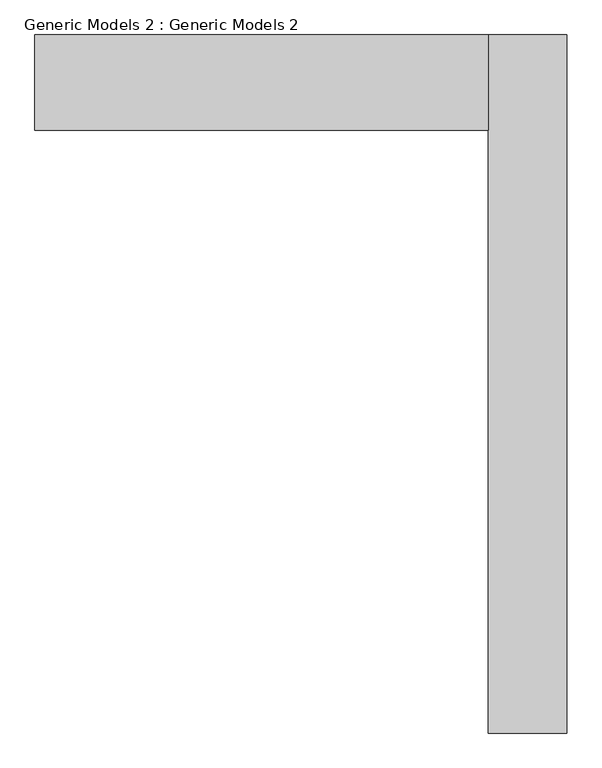
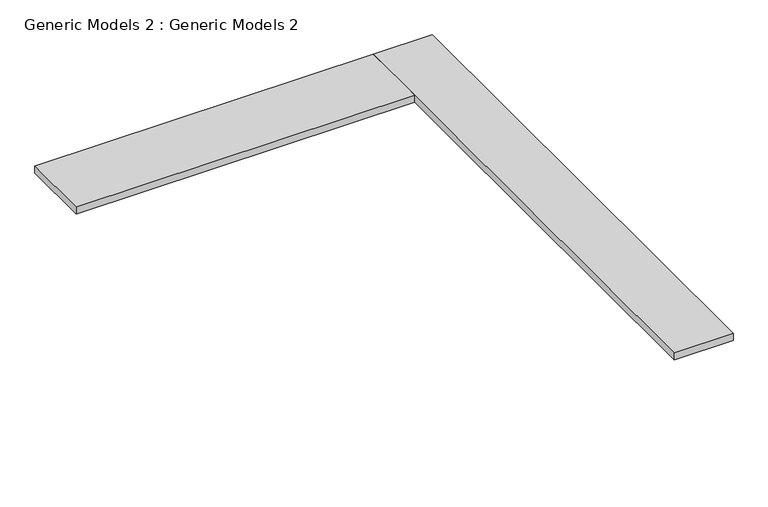
"""IFC4 building model written with IfcOpenShell, lengths in millimetres: proxy geometry, Generic Models 2 : Generic Models 2."""

from ifc_helpers import new_model, si_unit, frame, origin, place, context, project, spatial, polyline, outline, extrude, source, transform, mapped, element, save


def generic_models_2_generic_models_2_8981c4c3(model_context):
    return source(origin(), model_context, "Body", "SweptSolid", [
        extrude(outline(polyline([(-3848.1, 17233.2753534), (-3848.1, 20205.7), (10248.9, 20205.7), (10248.9, 17233.2753534), (-3848.1, 17233.2753534)])), frame((0.0, 0.0, -76.2), z_axis=(0.0, 0.0, 1.0), x_axis=(1.0, 0.0, 0.0)), (0.0, 0.0, 1.0), 304.8),
        extrude(outline(polyline([(12697.3223737, 20205.7), (12697.3223737, -1511.3), (10248.9, -1511.3), (10248.9, 20205.7), (12697.3223737, 20205.7)])), frame((0.0, 0.0, -76.2), z_axis=(0.0, 0.0, 1.0), x_axis=(1.0, 0.0, 0.0)), (0.0, 0.0, 1.0), 304.8),
    ])


if __name__ == "__main__":
    model = new_model("IFC4")
    model_context = context("Model", 3, world=origin())
    ifc_project = project(units=[si_unit("LENGTHUNIT", "METRE", prefix="MILLI")], contexts=[model_context])
    site = spatial("IfcSite", under=ifc_project)
    building = spatial("IfcBuilding", under=site)
    placement = place(None, origin())
    generic_models_2_generic_models_2_shape = generic_models_2_generic_models_2_8981c4c3(model_context)
    element("IfcBuildingElementProxy", 1, Name="Generic Models 2 : Generic Models 2", ObjectType="Generic Models 2 : Generic Models 2", at=placement, inside=building, context=model_context, shape_type="MappedRepresentation", body=[
        mapped(generic_models_2_generic_models_2_shape, transform((0.0, 0.0, 0.0), x_axis=(1.0, 0.0, 0.0), y_axis=(0.0, 1.0, 0.0), z_axis=(0.0, 0.0, 1.0))),
    ])
    save(model, "model.ifc")
